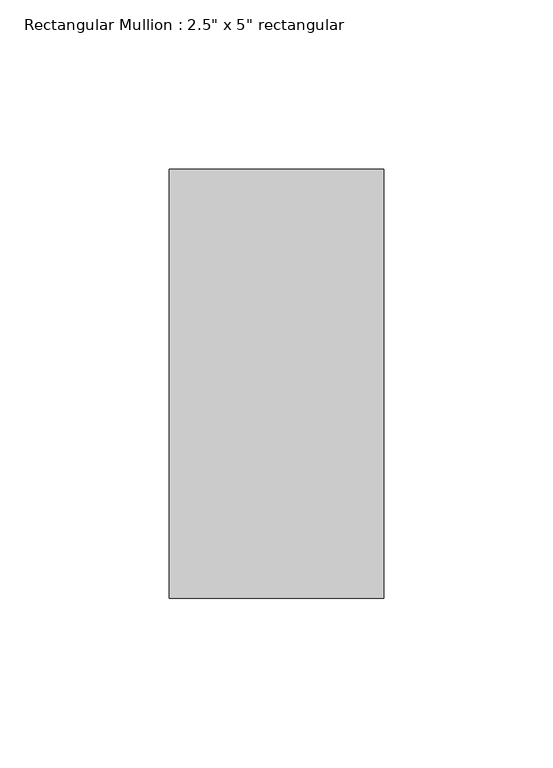
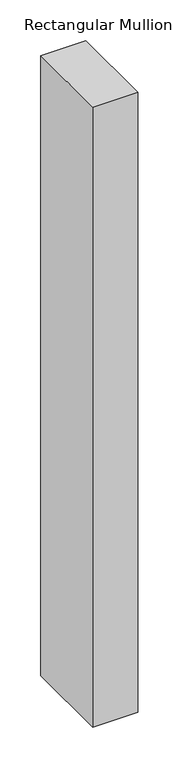
"""IFC4 building model written with IfcOpenShell, lengths in millimetres: member geometry."""

from ifc_helpers import new_model, si_unit, frame, origin, place, context, project, spatial, polyline, outline, extrude, source, transform, mapped, element, save


def member_846957be(model_context):
    return source(origin(), model_context, "Body", "SweptSolid", [
        extrude(outline(polyline([(31.75, 63.5), (31.75, -63.5), (-31.75, -63.5), (-31.75, 63.5), (31.75, 63.5)])), frame((0.0, 0.0, -925.9054943), z_axis=(0.0, 0.0, 1.0), x_axis=(1.0, 0.0, 0.0)), (0.0, 0.0, 1.0), 925.9054943),
    ])


if __name__ == "__main__":
    model = new_model("IFC4")
    model_context = context("Model", 3, world=origin())
    ifc_project = project(units=[si_unit("LENGTHUNIT", "METRE", prefix="MILLI")], contexts=[model_context])
    site = spatial("IfcSite", under=ifc_project)
    building = spatial("IfcBuilding", under=site)
    placement = place(None, origin())
    member_shape = member_846957be(model_context)
    element("IfcMember", 1, ObjectType="Rectangular Mullion : 2.5\" x 5\" rectangular", at=placement, inside=building, context=model_context, shape_type="MappedRepresentation", body=[
        mapped(member_shape, transform((0.0, 0.0, 0.0), x_axis=(1.0, 0.0, 0.0), y_axis=(0.0, 1.0, 0.0), z_axis=(0.0, 0.0, 1.0))),
    ])
    save(model, "model.ifc")

# Revit data of these elements
# Type "Rectangular Mullion : 2.5\" x 5\" rectangular"
#   built-in parameter 1007304 = 0.416667 (stored number, unit not read)
#   built-in parameter 1007301 = 0.104167 (stored number, unit not read)
#   built-in parameter 1007300 = 0.104167 (stored number, unit not read)
# Element 1 (IfcMember, "Rectangular Mullion : 2.5\" x 5\" rectangular")
#   Materials on its faces: "Aluminum"
# Materials
#   "Aluminum": class "Metal", colour RGB 247 247 247, transparency 0, Description = "Aluminum 6061", Cost = 0
